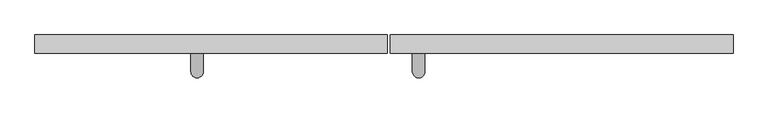
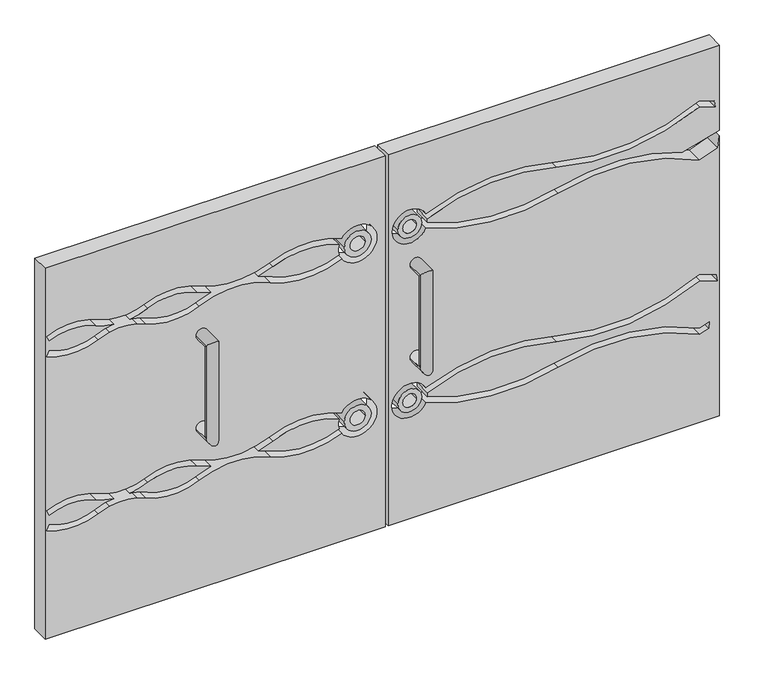
"""IFC4 building model written with IfcOpenShell, lengths in millimetres: proxy geometry."""

from ifc_helpers import new_model, si_unit, point, frame, frame_2d, origin, place, context, project, spatial, polyline, circle_curve, ellipse_curve, trimmed, segment, composite_curve, outline, extrude, source, transform, mapped, element, save
from ifc_brep_helpers import plane_surface, cylinder_surface, advanced_brep


def generic_models_a1fe0e04(model_context):
    return source(origin(), model_context, "Body", "SolidModel", [
        extrude(outline(polyline([(1676.4, 0.0), (1676.4, -1453.902355), (0.0, -1453.902355), (0.0, 0.0), (1676.4, 0.0)]), holes=[composite_curve([segment(trimmed(circle_curve(frame_2d((1702.6736745, -644.0023752)), 369.6247548), [point((1365.9294104, -796.4023752))], [point((1365.9294104, -491.6023752))], False, "CARTESIAN"), True, "CONTINUOUS"), segment(trimmed(circle_curve(frame_2d((1029.1851463, -339.2023752)), 369.6247548), [point((1365.9294104, -491.6023752))], [point((1365.9294104, -186.8023752))], True, "CARTESIAN"), True, "CONTINUOUS"), segment(trimmed(circle_curve(frame_2d((1320.8, -117.6804625)), 82.55), [point((1365.9294104, -186.8023752))], [point((1275.6705896, -186.8023752))], True, "CARTESIAN"), True, "CONTINUOUS"), segment(trimmed(circle_curve(frame_2d((1612.4148537, -339.2023752)), 369.6247548), [point((1275.6705896, -186.8023752))], [point((1275.6705896, -491.6023752))], True, "CARTESIAN"), True, "CONTINUOUS"), segment(trimmed(circle_curve(frame_2d((938.9263255, -644.0023752)), 369.6247548), [point((1275.6705896, -491.6023752))], [point((1275.6705896, -796.4023752))], False, "CARTESIAN"), True, "CONTINUOUS"), segment(trimmed(circle_curve(frame_2d((1528.2287877, -910.7023752)), 277.2185661), [point((1275.6705896, -796.4023752))], [point((1275.6705896, -1025.0023752))], True, "CARTESIAN"), True, "CONTINUOUS"), segment(trimmed(circle_curve(frame_2d((1051.1744135, -1126.6023752)), 246.4165032), [point((1275.6705896, -1025.0023752))], [point((1289.1262093, -1062.5708522))], False, "CARTESIAN"), True, "CONTINUOUS"), segment(trimmed(circle_curve(frame_2d((1051.1744135, -1126.6023752)), 246.4165032), [point((1289.1262093, -1062.5708522))], [point((1291.8650264, -1179.4145132))], False, "CARTESIAN"), True, "CONTINUOUS"), segment(trimmed(circle_curve(frame_2d((1051.1744135, -1126.6023752)), 246.4165032), [point((1291.8650264, -1179.4145132))], [point((1275.6705896, -1228.2023752))], False, "CARTESIAN"), True, "CONTINUOUS"), segment(trimmed(circle_curve(frame_2d((1518.2829274, -1338.0011876)), 266.301569), [point((1275.6705896, -1228.2023752))], [point((1275.6705896, -1447.8))], True, "CARTESIAN"), True, "CONTINUOUS"), segment(polyline([(1275.6705896, -1447.8), (1298.8110968, -1437.3273248)]), True, "CONTINUOUS"), segment(trimmed(circle_curve(frame_2d((1518.2829274, -1338.0011876)), 240.901569), [point((1298.8110968, -1437.3273248))], [point((1298.8110968, -1238.6750504))], False, "CARTESIAN"), True, "CONTINUOUS"), segment(trimmed(circle_curve(frame_2d((1051.1744135, -1126.6023752)), 271.8165032), [point((1298.8110968, -1238.6750504))], [point((1320.8, -1161.0444215))], True, "CARTESIAN"), True, "CONTINUOUS"), segment(trimmed(circle_curve(frame_2d((1590.4255865, -1126.6023752)), 271.8165032), [point((1320.8, -1161.0444215))], [point((1342.7889032, -1238.6750504))], True, "CARTESIAN"), True, "CONTINUOUS"), segment(trimmed(circle_curve(frame_2d((1123.3170726, -1338.0011876)), 240.901569), [point((1342.7889032, -1238.6750504))], [point((1342.7889032, -1437.3273248))], False, "CARTESIAN"), True, "CONTINUOUS"), segment(polyline([(1342.7889032, -1437.3273248), (1365.9294104, -1447.8)]), True, "CONTINUOUS"), segment(trimmed(circle_curve(frame_2d((1123.3170726, -1338.0011876)), 266.301569), [point((1365.9294104, -1447.8))], [point((1365.9294104, -1228.2023752))], True, "CARTESIAN"), True, "CONTINUOUS"), segment(trimmed(circle_curve(frame_2d((1590.4255865, -1126.6023752)), 246.4165032), [point((1365.9294104, -1228.2023752))], [point((1365.9294104, -1025.0023752))], False, "CARTESIAN"), True, "CONTINUOUS"), segment(trimmed(circle_curve(frame_2d((1113.3712123, -910.7023752)), 277.2185661), [point((1365.9294104, -1025.0023752))], [point((1365.9294104, -796.4023752))], True, "CARTESIAN"), True, "CONTINUOUS")], self_intersect=False), composite_curve([segment(trimmed(circle_curve(frame_2d((915.2736745, -644.0023752)), 369.6247548), [point((578.5294104, -796.4023752))], [point((578.5294104, -491.6023752))], False, "CARTESIAN"), True, "CONTINUOUS"), segment(trimmed(circle_curve(frame_2d((241.7851463, -339.2023752)), 369.6247548), [point((578.5294104, -491.6023752))], [point((578.5294104, -186.8023752))], True, "CARTESIAN"), True, "CONTINUOUS"), segment(trimmed(circle_curve(frame_2d((533.4, -117.6804625)), 82.55), [point((578.5294104, -186.8023752))], [point((488.2705896, -186.8023752))], True, "CARTESIAN"), True, "CONTINUOUS"), segment(trimmed(circle_curve(frame_2d((825.0148537, -339.2023752)), 369.6247548), [point((488.2705896, -186.8023752))], [point((488.2705896, -491.6023752))], True, "CARTESIAN"), True, "CONTINUOUS"), segment(trimmed(circle_curve(frame_2d((151.5263255, -644.0023752)), 369.6247548), [point((488.2705896, -491.6023752))], [point((488.2705896, -796.4023752))], False, "CARTESIAN"), True, "CONTINUOUS"), segment(trimmed(circle_curve(frame_2d((740.8287877, -910.7023752)), 277.2185661), [point((488.2705896, -796.4023752))], [point((488.2705896, -1025.0023752))], True, "CARTESIAN"), True, "CONTINUOUS"), segment(trimmed(circle_curve(frame_2d((263.7744135, -1126.6023752)), 246.4165032), [point((488.2705896, -1025.0023752))], [point((501.7262093, -1062.5708522))], False, "CARTESIAN"), True, "CONTINUOUS"), segment(trimmed(circle_curve(frame_2d((263.7744135, -1126.6023752)), 246.4165032), [point((501.7262093, -1062.5708522))], [point((504.4650264, -1179.4145132))], False, "CARTESIAN"), True, "CONTINUOUS"), segment(trimmed(circle_curve(frame_2d((263.7744135, -1126.6023752)), 246.4165032), [point((504.4650264, -1179.4145132))], [point((488.2705896, -1228.2023752))], False, "CARTESIAN"), True, "CONTINUOUS"), segment(trimmed(circle_curve(frame_2d((730.8829274, -1338.0011876)), 266.301569), [point((488.2705896, -1228.2023752))], [point((488.2705896, -1447.8))], True, "CARTESIAN"), True, "CONTINUOUS"), segment(polyline([(488.2705896, -1447.8), (511.4110968, -1437.3273248)]), True, "CONTINUOUS"), segment(trimmed(circle_curve(frame_2d((730.8829274, -1338.0011876)), 240.901569), [point((511.4110968, -1437.3273248))], [point((511.4110968, -1238.6750504))], False, "CARTESIAN"), True, "CONTINUOUS"), segment(trimmed(circle_curve(frame_2d((263.7744135, -1126.6023752)), 271.8165032), [point((511.4110968, -1238.6750504))], [point((533.4, -1161.0444215))], True, "CARTESIAN"), True, "CONTINUOUS"), segment(trimmed(circle_curve(frame_2d((803.0255865, -1126.6023752)), 271.8165032), [point((533.4, -1161.0444215))], [point((555.3889032, -1238.6750504))], True, "CARTESIAN"), True, "CONTINUOUS"), segment(trimmed(circle_curve(frame_2d((335.9170726, -1338.0011876)), 240.901569), [point((555.3889032, -1238.6750504))], [point((555.3889032, -1437.3273248))], False, "CARTESIAN"), True, "CONTINUOUS"), segment(polyline([(555.3889032, -1437.3273248), (578.5294104, -1447.8)]), True, "CONTINUOUS"), segment(trimmed(circle_curve(frame_2d((335.9170726, -1338.0011876)), 266.301569), [point((578.5294104, -1447.8))], [point((578.5294104, -1228.2023752))], True, "CARTESIAN"), True, "CONTINUOUS"), segment(trimmed(circle_curve(frame_2d((803.0255865, -1126.6023752)), 246.4165032), [point((578.5294104, -1228.2023752))], [point((578.5294104, -1025.0023752))], False, "CARTESIAN"), True, "CONTINUOUS"), segment(trimmed(circle_curve(frame_2d((325.9712123, -910.7023752)), 277.2185661), [point((578.5294104, -1025.0023752))], [point((578.5294104, -796.4023752))], True, "CARTESIAN"), True, "CONTINUOUS")], self_intersect=False)]), frame((0.0, -76.2, 0.0), z_axis=(0.0, 1.0, 0.0), x_axis=(0.0, 0.0, 1.0)), (0.0, 0.0, 1.0), 76.2),
        extrude(outline(composite_curve([segment(polyline([(1676.4, 1428.9981988), (1676.4, 12.7), (0.0, 12.7), (0.0, 1428.9981988), (1265.6077639, 1428.9981988), (1213.8226002, 1422.0502947)]), True, "CONTINUOUS"), segment(trimmed(circle_curve(frame_2d((18.1783659, 1806.9541317)), 1256.0716933), [point((1213.8226002, 1422.0502947))], [point((1185.7081212, 1343.7151338))], False, "CARTESIAN"), True, "CONTINUOUS"), segment(trimmed(circle_curve(frame_2d((454.8711686, 960.4221512)), 825.2491514), [point((1185.7081212, 1343.7151338))], [point((1249.4286724, 737.4545864))], False, "CARTESIAN"), True, "CONTINUOUS"), segment(trimmed(circle_curve(frame_2d((2064.057677, 508.8545864)), 846.0959609), [point((1249.4286724, 737.4545864))], [point((1287.4409925, 173.0795121))], True, "CARTESIAN"), True, "CONTINUOUS"), segment(trimmed(circle_curve(frame_2d((1320.8, 104.5695375)), 76.2), [point((1287.4409925, 173.0795121))], [point((1354.1590075, 173.0795121))], True, "CARTESIAN"), True, "CONTINUOUS"), segment(trimmed(circle_curve(frame_2d((577.542323, 508.8545864)), 846.0959609), [point((1354.1590075, 173.0795121))], [point((1392.1713276, 737.4545864))], True, "CARTESIAN"), True, "CONTINUOUS"), segment(trimmed(circle_curve(frame_2d((2186.7288314, 960.4221512)), 825.2491514), [point((1392.1713276, 737.4545864))], [point((1455.8918788, 1343.7151338))], False, "CARTESIAN"), True, "CONTINUOUS"), segment(trimmed(circle_curve(frame_2d((2623.4216341, 1806.9541317)), 1256.0716933), [point((1455.8918788, 1343.7151338))], [point((1432.8106543, 1406.7521908))], False, "CARTESIAN"), True, "CONTINUOUS"), segment(polyline([(1432.8106543, 1406.7521908), (1404.8157377, 1410.5082086)]), True, "CONTINUOUS"), segment(trimmed(circle_curve(frame_2d((2623.4216341, 1806.9541317)), 1281.4716933), [point((1404.8157377, 1410.5082086))], [point((1428.0530461, 1345.1493682))], True, "CARTESIAN"), True, "CONTINUOUS"), segment(trimmed(circle_curve(frame_2d((2186.7288314, 960.4221512)), 850.6491514), [point((1428.0530461, 1345.1493682))], [point((1367.7159731, 730.5919605))], True, "CARTESIAN"), True, "CONTINUOUS"), segment(trimmed(circle_curve(frame_2d((577.542323, 508.8545864)), 820.6959609), [point((1367.7159731, 730.5919605))], [point((1329.5851361, 180.261422))], False, "CARTESIAN"), True, "CONTINUOUS"), segment(trimmed(circle_curve(frame_2d((1320.8, 104.5695375)), 76.2), [point((1329.5851361, 180.261422))], [point((1312.0148639, 180.261422))], True, "CARTESIAN"), True, "CONTINUOUS"), segment(trimmed(circle_curve(frame_2d((2064.057677, 508.8545864)), 820.6959609), [point((1312.0148639, 180.261422))], [point((1273.8840269, 730.5919605))], False, "CARTESIAN"), True, "CONTINUOUS"), segment(trimmed(circle_curve(frame_2d((454.8711686, 960.4221512)), 850.6491514), [point((1273.8840269, 730.5919605))], [point((1247.3512879, 1269.5810733))], True, "CARTESIAN"), True, "CONTINUOUS"), segment(trimmed(circle_curve(frame_2d((35.6048011, 1686.5224988)), 1281.4716933), [point((1247.3512879, 1269.5810733))], [point((1290.9338159, 1428.9981988))], True, "CARTESIAN"), True, "CONTINUOUS"), segment(polyline([(1290.9338159, 1428.9981988), (1676.4, 1428.9981988)]), True, "CONTINUOUS")], self_intersect=False), holes=[composite_curve([segment(trimmed(circle_curve(frame_2d((1399.3288314, 960.4221512)), 825.2491514), [point((604.7713276, 737.4545864))], [point((668.4918788, 1343.7151338))], False, "CARTESIAN"), True, "CONTINUOUS"), segment(trimmed(circle_curve(frame_2d((1836.0216341, 1806.9541317)), 1256.0716933), [point((668.4918788, 1343.7151338))], [point((642.1307432, 1416.6457417))], False, "CARTESIAN"), True, "CONTINUOUS"), segment(polyline([(642.1307432, 1416.6457417), (614.2460701, 1420.3869683)]), True, "CONTINUOUS"), segment(trimmed(circle_curve(frame_2d((1836.0216341, 1806.9541317)), 1281.4716933), [point((614.2460701, 1420.3869683))], [point((640.6530461, 1345.1493682))], True, "CARTESIAN"), True, "CONTINUOUS"), segment(trimmed(circle_curve(frame_2d((1399.3288314, 960.4221512)), 850.6491514), [point((640.6530461, 1345.1493682))], [point((580.3159731, 730.5919605))], True, "CARTESIAN"), True, "CONTINUOUS"), segment(trimmed(circle_curve(frame_2d((-209.857677, 508.8545864)), 820.6959609), [point((580.3159731, 730.5919605))], [point((542.1851361, 180.261422))], False, "CARTESIAN"), True, "CONTINUOUS"), segment(trimmed(circle_curve(frame_2d((533.4, 104.5695375)), 76.2), [point((542.1851361, 180.261422))], [point((524.6148639, 180.261422))], True, "CARTESIAN"), True, "CONTINUOUS"), segment(trimmed(circle_curve(frame_2d((1276.657677, 508.8545864)), 820.6959609), [point((524.6148639, 180.261422))], [point((486.4840269, 730.5919605))], False, "CARTESIAN"), True, "CONTINUOUS"), segment(trimmed(circle_curve(frame_2d((-332.5288314, 960.4221512)), 850.6491514), [point((486.4840269, 730.5919605))], [point((426.1469539, 1345.1493682))], True, "CARTESIAN"), True, "CONTINUOUS"), segment(trimmed(circle_curve(frame_2d((-769.2216341, 1806.9541317)), 1281.4716933), [point((426.1469539, 1345.1493682))], [point((441.3119434, 1386.5041841))], True, "CARTESIAN"), True, "CONTINUOUS"), segment(polyline([(441.3119434, 1386.5041841), (413.0361304, 1382.7104791)]), True, "CONTINUOUS"), segment(trimmed(circle_curve(frame_2d((-769.2216341, 1806.9541317)), 1256.0716933), [point((413.0361304, 1382.7104791))], [point((398.3081212, 1343.7151338))], False, "CARTESIAN"), True, "CONTINUOUS"), segment(trimmed(circle_curve(frame_2d((-332.5288314, 960.4221512)), 825.2491514), [point((398.3081212, 1343.7151338))], [point((462.0286724, 737.4545864))], False, "CARTESIAN"), True, "CONTINUOUS"), segment(trimmed(circle_curve(frame_2d((1276.657677, 508.8545864)), 846.0959609), [point((462.0286724, 737.4545864))], [point((500.0409925, 173.0795121))], True, "CARTESIAN"), True, "CONTINUOUS"), segment(trimmed(circle_curve(frame_2d((533.4, 104.5695375)), 76.2), [point((500.0409925, 173.0795121))], [point((566.7590075, 173.0795121))], True, "CARTESIAN"), True, "CONTINUOUS"), segment(trimmed(circle_curve(frame_2d((-209.857677, 508.8545864)), 846.0959609), [point((566.7590075, 173.0795121))], [point((604.7713276, 737.4545864))], True, "CARTESIAN"), True, "CONTINUOUS")], self_intersect=False)]), frame((0.0, -76.2, 0.0), z_axis=(0.0, 1.0, 0.0), x_axis=(0.0, 0.0, 1.0)), (0.0, 0.0, 1.0), 76.2),
        extrude(outline(composite_curve([segment(trimmed(circle_curve(frame_2d((1612.4148537, -339.2023752)), 344.2247548), [point((1298.8110968, -481.1297))], [point((1298.8219854, -197.2509933))], False, "CARTESIAN"), True, "CONTINUOUS"), segment(trimmed(circle_curve(frame_2d((1320.8, -117.6804625)), 82.55), [point((1298.8219854, -197.2509933))], [point((1342.7780146, -197.2509933))], True, "CARTESIAN"), True, "CONTINUOUS"), segment(trimmed(circle_curve(frame_2d((1029.1851463, -339.2023752)), 344.2247548), [point((1342.7780146, -197.2509933))], [point((1342.7889032, -481.1297))], False, "CARTESIAN"), True, "CONTINUOUS"), segment(trimmed(circle_curve(frame_2d((1702.6736745, -644.0023752)), 395.0247548), [point((1342.7889032, -481.1297))], [point((1320.8, -542.9229328))], True, "CARTESIAN"), True, "CONTINUOUS"), segment(trimmed(circle_curve(frame_2d((938.9263255, -644.0023752)), 395.0247548), [point((1320.8, -542.9229328))], [point((1298.8110968, -481.1297))], True, "CARTESIAN"), True, "CONTINUOUS")], self_intersect=False)), frame((0.0, -76.2, 0.0), z_axis=(0.0, 1.0, 0.0), x_axis=(0.0, 0.0, 1.0)), (0.0, 0.0, 1.0), 76.2),
        extrude(outline(composite_curve([segment(trimmed(circle_curve(frame_2d((1320.8, -117.6804625)), 57.15), [point((1320.8, -174.8304625))], [point((1320.8, -60.5304625))], False, "CARTESIAN"), True, "CONTINUOUS"), segment(trimmed(circle_curve(frame_2d((1320.8, -117.6804625)), 57.15), [point((1320.8, -60.5304625))], [point((1320.8, -174.8304625))], False, "CARTESIAN"), True, "CONTINUOUS")], self_intersect=False), holes=[composite_curve([segment(trimmed(circle_curve(frame_2d((1320.8, -117.6804625)), 31.75), [point((1320.8, -149.4304625))], [point((1320.8, -85.9304625))], True, "CARTESIAN"), True, "CONTINUOUS"), segment(trimmed(circle_curve(frame_2d((1320.8, -117.6804625)), 31.75), [point((1320.8, -85.9304625))], [point((1320.8, -149.4304625))], True, "CARTESIAN"), True, "CONTINUOUS")], self_intersect=False)]), frame((0.0, -76.2, 0.0), z_axis=(0.0, 1.0, 0.0), x_axis=(0.0, 0.0, 1.0)), (0.0, 0.0, 1.0), 76.2),
        extrude(outline(composite_curve([segment(trimmed(circle_curve(frame_2d((1113.3712123, -910.7023752)), 251.8185661), [point((1342.7889032, -806.8750504))], [point((1342.7889032, -1014.5297))], False, "CARTESIAN"), True, "CONTINUOUS"), segment(trimmed(circle_curve(frame_2d((1590.4255865, -1126.6023752)), 271.8165032), [point((1342.7889032, -1014.5297))], [point((1320.8, -1092.1603289))], True, "CARTESIAN"), True, "CONTINUOUS"), segment(trimmed(circle_curve(frame_2d((1051.1744135, -1126.6023752)), 271.8165032), [point((1320.8, -1092.1603289))], [point((1298.8110968, -1014.5297))], True, "CARTESIAN"), True, "CONTINUOUS"), segment(trimmed(circle_curve(frame_2d((1528.2287877, -910.7023752)), 251.8185661), [point((1298.8110968, -1014.5297))], [point((1298.8110968, -806.8750504))], False, "CARTESIAN"), True, "CONTINUOUS"), segment(trimmed(circle_curve(frame_2d((938.9263255, -644.0023752)), 395.0247548), [point((1298.8110968, -806.8750504))], [point((1320.8, -745.0818176))], True, "CARTESIAN"), True, "CONTINUOUS"), segment(trimmed(circle_curve(frame_2d((1702.6736745, -644.0023752)), 395.0247548), [point((1320.8, -745.0818176))], [point((1342.7889032, -806.8750504))], True, "CARTESIAN"), True, "CONTINUOUS")], self_intersect=False)), frame((0.0, -76.2, 0.0), z_axis=(0.0, 1.0, 0.0), x_axis=(0.0, 0.0, 1.0)), (0.0, 0.0, 1.0), 76.2),
        extrude(outline(composite_curve([segment(trimmed(circle_curve(frame_2d((825.0148537, -339.2023752)), 344.2247548), [point((511.4110968, -481.1297))], [point((511.4219854, -197.2509933))], False, "CARTESIAN"), True, "CONTINUOUS"), segment(trimmed(circle_curve(frame_2d((533.4, -117.6804625)), 82.55), [point((511.4219854, -197.2509933))], [point((555.3780146, -197.2509933))], True, "CARTESIAN"), True, "CONTINUOUS"), segment(trimmed(circle_curve(frame_2d((241.7851463, -339.2023752)), 344.2247548), [point((555.3780146, -197.2509933))], [point((555.3889032, -481.1297))], False, "CARTESIAN"), True, "CONTINUOUS"), segment(trimmed(circle_curve(frame_2d((915.2736745, -644.0023752)), 395.0247548), [point((555.3889032, -481.1297))], [point((533.4, -542.9229328))], True, "CARTESIAN"), True, "CONTINUOUS"), segment(trimmed(circle_curve(frame_2d((151.5263255, -644.0023752)), 395.0247548), [point((533.4, -542.9229328))], [point((511.4110968, -481.1297))], True, "CARTESIAN"), True, "CONTINUOUS")], self_intersect=False)), frame((0.0, -76.2, 0.0), z_axis=(0.0, 1.0, 0.0), x_axis=(0.0, 0.0, 1.0)), (0.0, 0.0, 1.0), 76.2),
        extrude(outline(composite_curve([segment(trimmed(circle_curve(frame_2d((533.4, -117.6804625)), 57.15), [point((533.4, -174.8304625))], [point((533.4, -60.5304625))], False, "CARTESIAN"), True, "CONTINUOUS"), segment(trimmed(circle_curve(frame_2d((533.4, -117.6804625)), 57.15), [point((533.4, -60.5304625))], [point((533.4, -174.8304625))], False, "CARTESIAN"), True, "CONTINUOUS")], self_intersect=False), holes=[composite_curve([segment(trimmed(circle_curve(frame_2d((533.4, -117.6804625)), 31.75), [point((533.4, -149.4304625))], [point((533.4, -85.9304625))], True, "CARTESIAN"), True, "CONTINUOUS"), segment(trimmed(circle_curve(frame_2d((533.4, -117.6804625)), 31.75), [point((533.4, -85.9304625))], [point((533.4, -149.4304625))], True, "CARTESIAN"), True, "CONTINUOUS")], self_intersect=False)]), frame((0.0, -76.2, 0.0), z_axis=(0.0, 1.0, 0.0), x_axis=(0.0, 0.0, 1.0)), (0.0, 0.0, 1.0), 76.2),
        extrude(outline(composite_curve([segment(trimmed(circle_curve(frame_2d((325.9712123, -910.7023752)), 251.8185661), [point((555.3889032, -806.8750504))], [point((555.3889032, -1014.5297))], False, "CARTESIAN"), True, "CONTINUOUS"), segment(trimmed(circle_curve(frame_2d((803.0255865, -1126.6023752)), 271.8165032), [point((555.3889032, -1014.5297))], [point((533.4, -1092.1603289))], True, "CARTESIAN"), True, "CONTINUOUS"), segment(trimmed(circle_curve(frame_2d((263.7744135, -1126.6023752)), 271.8165032), [point((533.4, -1092.1603289))], [point((511.4110968, -1014.5297))], True, "CARTESIAN"), True, "CONTINUOUS"), segment(trimmed(circle_curve(frame_2d((740.8287877, -910.7023752)), 251.8185661), [point((511.4110968, -1014.5297))], [point((511.4110968, -806.8750504))], False, "CARTESIAN"), True, "CONTINUOUS"), segment(trimmed(circle_curve(frame_2d((151.5263255, -644.0023752)), 395.0247548), [point((511.4110968, -806.8750504))], [point((533.4, -745.0818176))], True, "CARTESIAN"), True, "CONTINUOUS"), segment(trimmed(circle_curve(frame_2d((915.2736745, -644.0023752)), 395.0247548), [point((533.4, -745.0818176))], [point((555.3889032, -806.8750504))], True, "CARTESIAN"), True, "CONTINUOUS")], self_intersect=False)), frame((0.0, -76.2, 0.0), z_axis=(0.0, 1.0, 0.0), x_axis=(0.0, 0.0, 1.0)), (0.0, 0.0, 1.0), 76.2),
        extrude(outline(composite_curve([segment(trimmed(circle_curve(frame_2d((1320.8, 104.5695375)), 50.8), [point((1320.8, 53.7695375))], [point((1320.8, 155.3695375))], False, "CARTESIAN"), True, "CONTINUOUS"), segment(trimmed(circle_curve(frame_2d((1320.8, 104.5695375)), 50.8), [point((1320.8, 155.3695375))], [point((1320.8, 53.7695375))], False, "CARTESIAN"), True, "CONTINUOUS")], self_intersect=False), holes=[composite_curve([segment(trimmed(circle_curve(frame_2d((1320.8, 104.5695375)), 29.0480022), [point((1320.8, 75.5215353))], [point((1320.8, 133.6175397))], True, "CARTESIAN"), True, "CONTINUOUS"), segment(trimmed(circle_curve(frame_2d((1320.8, 104.5695375)), 29.0480022), [point((1320.8, 133.6175397))], [point((1320.8, 75.5215353))], True, "CARTESIAN"), True, "CONTINUOUS")], self_intersect=False)]), frame((0.0, -76.2, 0.0), z_axis=(0.0, 1.0, 0.0), x_axis=(0.0, 0.0, 1.0)), (0.0, 0.0, 1.0), 76.2),
        extrude(outline(composite_curve([segment(trimmed(circle_curve(frame_2d((533.4, 104.5695375)), 50.8), [point((533.4, 53.7695375))], [point((533.4, 155.3695375))], False, "CARTESIAN"), True, "CONTINUOUS"), segment(trimmed(circle_curve(frame_2d((533.4, 104.5695375)), 50.8), [point((533.4, 155.3695375))], [point((533.4, 53.7695375))], False, "CARTESIAN"), True, "CONTINUOUS")], self_intersect=False), holes=[composite_curve([segment(trimmed(circle_curve(frame_2d((533.4, 104.5695375)), 29.0480022), [point((533.4, 75.5215353))], [point((533.4, 133.6175397))], True, "CARTESIAN"), True, "CONTINUOUS"), segment(trimmed(circle_curve(frame_2d((533.4, 104.5695375)), 29.0480022), [point((533.4, 133.6175397))], [point((533.4, 75.5215353))], True, "CARTESIAN"), True, "CONTINUOUS")], self_intersect=False)]), frame((0.0, -76.2, 0.0), z_axis=(0.0, 1.0, 0.0), x_axis=(0.0, 0.0, 1.0)), (0.0, 0.0, 1.0), 76.2),
        advanced_brep(
        [(-759.0077249, -75.5111086, 1145.6217371), (-809.8077249, -75.5111086, 1145.6217371), (-759.0077249, -151.7111086, 1145.6217371), (-809.8077249, -151.7111086, 1145.6217371), (-759.0077249, -151.7111086, 726.5217371), (-809.8077249, -151.7111086, 726.5217371), (-759.0077249, -75.5111086, 726.5217371), (-809.8077249, -75.5111086, 726.5217371)],
        [
            (0, 1, circle_curve(frame((-784.4077249, -75.5111086, 1145.6217371), z_axis=(0.0, 1.0, 0.0), x_axis=(-1.0, 0.0, 0.0)), 25.4)),
            (1, 0, circle_curve(frame((-784.4077249, -75.5111086, 1145.6217371), z_axis=(0.0, 1.0, 0.0), x_axis=(-1.0, 0.0, 0.0)), 25.4)),
            (0, 2),
            (2, 3, ellipse_curve(frame((-784.4077249, -151.7111086, 1145.6217371), z_axis=(0.0, 0.7071067811865502, 0.7071067811865448), x_axis=(0.0, 0.7071067811865448, -0.7071067811865501)), 35.9210245, 25.4)),
            (3, 1),
            (3, 2, ellipse_curve(frame((-784.4077249, -151.7111086, 1145.6217371), z_axis=(0.0, 0.7071067811865502, 0.7071067811865448), x_axis=(0.0, 0.7071067811865448, -0.7071067811865501)), 35.9210245, 25.4)),
            (2, 4),
            (4, 5, ellipse_curve(frame((-784.4077249, -151.7111086, 726.5217371), z_axis=(0.0, -0.7071067811865448, 0.7071067811865501), x_axis=(0.0, 0.70710678118655, 0.7071067811865451)), 35.9210245, 25.4)),
            (5, 3),
            (5, 4, ellipse_curve(frame((-784.4077249, -151.7111086, 726.5217371), z_axis=(0.0, -0.7071067811865448, 0.7071067811865501), x_axis=(0.0, 0.70710678118655, 0.7071067811865451)), 35.9210245, 25.4)),
            (6, 7, circle_curve(frame((-784.4077249, -75.5111086, 726.5217371), z_axis=(0.0, 1.0, 0.0), x_axis=(-1.0, 0.0, 0.0)), 25.4)),
            (7, 6, circle_curve(frame((-784.4077249, -75.5111086, 726.5217371), z_axis=(0.0, 1.0, 0.0), x_axis=(-1.0, 0.0, 0.0)), 25.4)),
            (4, 6),
            (7, 5),
        ],
        [
            plane_surface(frame((1428.9981988, -75.5111086, 1145.6217371), z_axis=(0.0, 1.0, 0.0), x_axis=(1.0, 0.0, 0.0))),
            cylinder_surface(frame((-784.4077249, -75.5111086, 1145.6217371), z_axis=(0.0, 1.0, 0.0), x_axis=(-1.0, 0.0, 0.0)), 25.4),
            cylinder_surface(frame((-784.4077249, -151.7111086, 1145.6217371), z_axis=(0.0, 0.0, 1.0), x_axis=(-1.0, 0.0, 0.0)), 25.4),
            plane_surface(frame((1428.9981988, -75.5111086, 726.5217371), z_axis=(0.0, 1.0, 0.0), x_axis=(1.0, 0.0, 0.0))),
            cylinder_surface(frame((-784.4077249, -151.7111086, 726.5217371), z_axis=(0.0, -1.0, 0.0), x_axis=(-1.0, 0.0, 0.0)), 25.4),
        ],
        [
            (0, [[1, 2]]),
            (1, [[-1, 3, 4, 5]]),
            (1, [[-2, -5, 6, -3]]),
            (2, [[-4, 7, 8, 9]]),
            (2, [[-6, -9, 10, -7]]),
            (3, [[11, 12]]),
            (4, [[-8, 13, -12, 14]]),
            (4, [[-10, -14, -11, -13]]),
        ],
    ),
        advanced_brep(
        [(105.2059236, -76.2192005, 1145.6217371), (156.0059236, -76.2192005, 1145.6217371), (156.0059236, -152.4192005, 1145.6217371), (105.2059236, -152.4192005, 1145.6217371), (156.0059236, -152.4192005, 726.5217371), (105.2059236, -152.4192005, 726.5217371), (105.2059236, -76.2192005, 726.5217371), (156.0059236, -76.2192005, 726.5217371)],
        [
            (0, 1, circle_curve(frame((130.6059236, -76.2192005, 1145.6217371), z_axis=(0.0, 1.0, 0.0), x_axis=(1.0, 0.0, 0.0)), 25.4)),
            (1, 0, circle_curve(frame((130.6059236, -76.2192005, 1145.6217371), z_axis=(0.0, 1.0, 0.0), x_axis=(1.0, 0.0, 0.0)), 25.4)),
            (1, 2),
            (2, 3, ellipse_curve(frame((130.6059236, -152.4192005, 1145.6217371), z_axis=(0.0, 0.7071067811865502, 0.7071067811865448), x_axis=(0.0, 0.7071067811865448, -0.7071067811865501)), 35.9210245, 25.4)),
            (3, 0),
            (3, 2, ellipse_curve(frame((130.6059236, -152.4192005, 1145.6217371), z_axis=(0.0, 0.7071067811865502, 0.7071067811865448), x_axis=(0.0, 0.7071067811865448, -0.7071067811865501)), 35.9210245, 25.4)),
            (2, 4),
            (4, 5, ellipse_curve(frame((130.6059236, -152.4192005, 726.5217371), z_axis=(0.0, -0.7071067811865448, 0.7071067811865501), x_axis=(0.0, 0.70710678118655, 0.7071067811865451)), 35.9210245, 25.4)),
            (5, 3),
            (5, 4, ellipse_curve(frame((130.6059236, -152.4192005, 726.5217371), z_axis=(0.0, -0.7071067811865448, 0.7071067811865501), x_axis=(0.0, 0.70710678118655, 0.7071067811865451)), 35.9210245, 25.4)),
            (6, 7, circle_curve(frame((130.6059236, -76.2192005, 726.5217371), z_axis=(0.0, 1.0, 0.0), x_axis=(1.0, 0.0, 0.0)), 25.4)),
            (7, 6, circle_curve(frame((130.6059236, -76.2192005, 726.5217371), z_axis=(0.0, 1.0, 0.0), x_axis=(1.0, 0.0, 0.0)), 25.4)),
            (4, 7),
            (6, 5),
        ],
        [
            plane_surface(frame((-2082.8, -76.2192005, 1145.6217371), z_axis=(0.0, 1.0, 0.0), x_axis=(-1.0, 0.0, 0.0))),
            cylinder_surface(frame((130.6059236, -76.2192005, 1145.6217371), z_axis=(0.0, 1.0, 0.0), x_axis=(1.0, 0.0, 0.0)), 25.4),
            cylinder_surface(frame((130.6059236, -152.4192005, 1145.6217371), z_axis=(0.0, 0.0, 1.0), x_axis=(1.0, 0.0, 0.0)), 25.4),
            plane_surface(frame((-2082.8, -76.2192005, 726.5217371), z_axis=(0.0, 1.0, 0.0), x_axis=(-1.0, 0.0, 0.0))),
            cylinder_surface(frame((130.6059236, -152.4192005, 726.5217371), z_axis=(0.0, -1.0, 0.0), x_axis=(1.0, 0.0, 0.0)), 25.4),
        ],
        [
            (0, [[1, 2]]),
            (1, [[-2, 3, 4, 5]]),
            (1, [[-1, -5, 6, -3]]),
            (2, [[-4, 7, 8, 9]]),
            (2, [[-6, -9, 10, -7]]),
            (3, [[11, 12]]),
            (4, [[-8, 13, -11, 14]]),
            (4, [[-10, -14, -12, -13]]),
        ],
    ),
    ])


if __name__ == "__main__":
    model = new_model("IFC4")
    model_context = context("Model", 3, world=origin())
    ifc_project = project(units=[si_unit("LENGTHUNIT", "METRE", prefix="MILLI")], contexts=[model_context])
    site = spatial("IfcSite", under=ifc_project)
    building = spatial("IfcBuilding", under=site)
    placement = place(None, origin())
    generic_models_shape = generic_models_a1fe0e04(model_context)
    element("IfcBuildingElementProxy", 1, Name="Generic Models", at=placement, inside=building, context=model_context, shape_type="MappedRepresentation", body=[
        mapped(generic_models_shape, transform((0.0, 0.0, 0.0), x_axis=(1.0, 0.0, 0.0), y_axis=(0.0, 1.0, 0.0), z_axis=(0.0, 0.0, 1.0))),
    ])
    save(model, "model.ifc")

# Revit data of these elements
# Type
#   Default Elevation = 0
# Element 1 (IfcBuildingElementProxy)
#   Materials on its faces: "GATE"
# Materials
#   "GATE": class "Generic", colour RGB 120 120 120, transparency 0, Cost = 0
